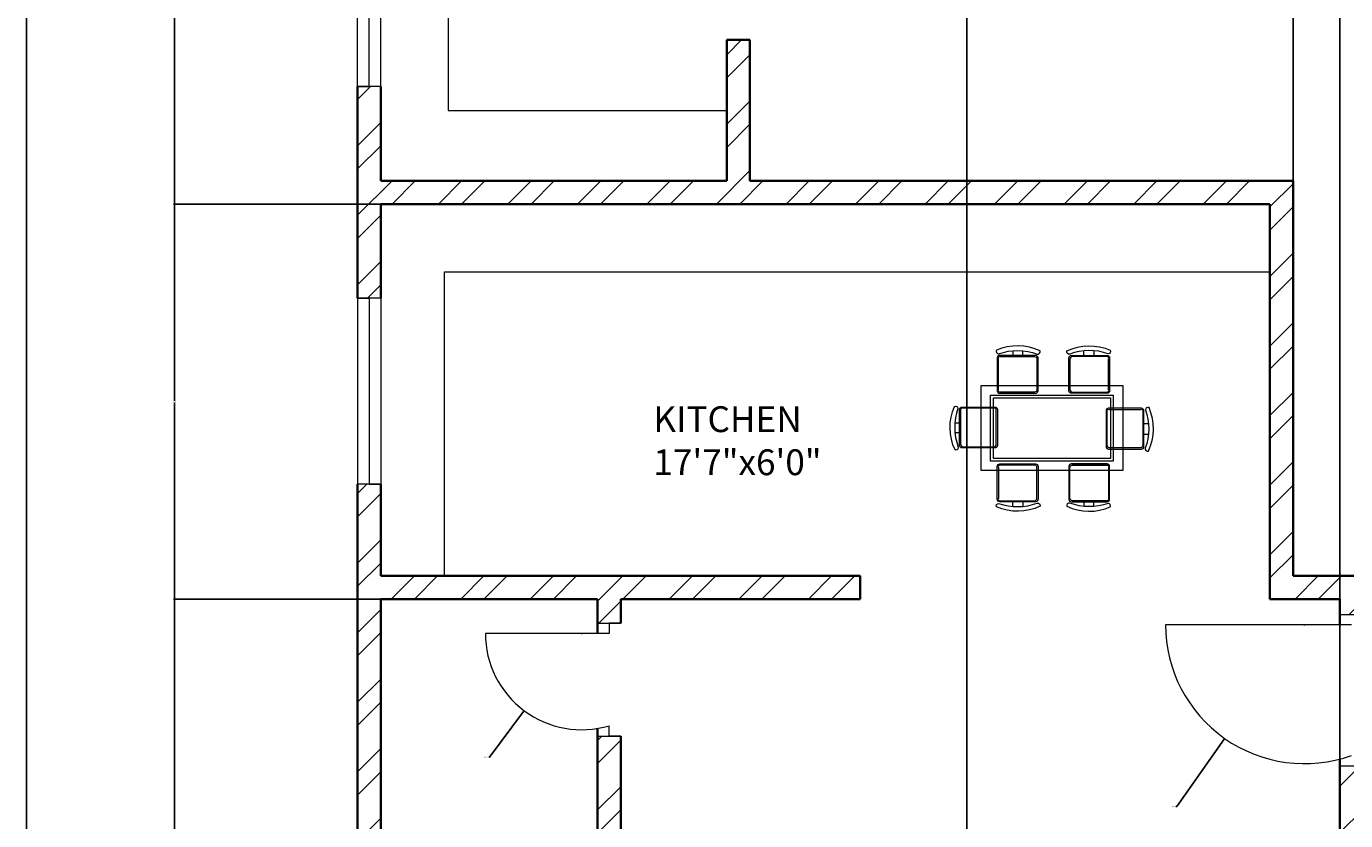
# Model space of a CAD drawing. Units: inches. Extents: x 2064 to 2782, y 1196 to 2299.
# Tile 3 of 11: x 2064 to 2320, y 1809 to 1963. Entities that reach past the tile are written whole.
import ezdxf

# ---------------------------------------------------------------- set-up
doc = ezdxf.new("R2010")
doc.units = ezdxf.units.IN
for name, color, linetype, lineweight in [('A-ANNO-DIMS', 2, 'Continuous', 18), ('A-ANNO-TTLB', 7, 'Continuous', 25), ('A-AREA-IDEN', 7, 'Continuous', 18), ('A-DOOR', 11, 'Continuous', 18), ('A-FLOR-CASE', 8, 'Continuous', 18), ('A-FURN', 8, 'Continuous', 13), ('A-GLAZ', 151, 'Continuous', 18), ('A-WALL', 7, 'Continuous', 35), ('A-WALL-PATT', 9, 'Continuous', 13)]:
    doc.layers.add(name, color=color, linetype=linetype, lineweight=lineweight)
doc.styles.get("Standard").update_dxf_attribs({"font": 'arial.ttf'})
doc.dimstyles.get("Standard").update_dxf_attribs({"dimtxt": 0.18, "dimasz": 0.18, "dimexe": 0.18, "dimexo": 0.0625, "dimgap": 0.09, "dimtad": 0, "dimtih": 1, "dimtoh": 1, "dimdec": 4, "dimzin": 0, "dimdsep": 46, "dimtxsty": 'Standard', "dimcen": 0.09, "dimadec": 0, "dimazin": 0, "dimtfac": 1, "dimtdec": 4, "dimtofl": 0, "dimtmove": 0, "dimatfit": 3, "dimfxl": 1, "dimtolj": 1, "dimtzin": 0, "dimarcsym": 0})

# ---------------------------------------------------------------- blocks, each defined once
blk = doc.blocks.new('WIN-36IN')
for p, q in [((0, 36), (4.5, 36)), ((0, 36), (0, 0)), ((4.5, 36), (2.25, 36)), ((2.25, 36), (2.25, 0)), ((4.5, 36), (4.5, 0)), ((2.25, 0), (0, 0)), ((0, 0), (4.5, 0))]:
    blk.add_line(p, q)
blk = doc.blocks.new('CHAIR-DINING')
for points in [[(7.35, 7.85, 0.414214), (6.87, 8.33), (0.49, 8.33, 0.414214), (0, 7.85), (0, 0.91, 0.414214), (0.49, 0.42), (6.87, 0.42, 0.414214), (7.35, 0.91), (7.35, 7.85)], [(7.35, 7.85, 0.414214), (6.87, 8.33), (0.49, 8.33, 0.414214), (0, 7.85), (0, 0.91, 0.414214), (0.49, 0.42), (6.87, 0.42, 0.414214), (7.35, 0.91), (7.35, 7.85)], [(7.65, 8.06, -0.175809), (7.6, 0.59, 0.578392), (8.22, 0.02, 0.214524), (8.33, 8.46, 0.552014), (7.65, 8.06, -0.065079)], [(7.65, 8.06, -0.175809), (7.6, 0.59, 0.578392), (8.22, 0.02, 0.214524), (8.33, 8.46, 0.552014), (7.65, 8.06, -0.065079)], [(7.35, 3.34), (8.23, 3.34, -0.064759)], [(7.35, 3.34), (8.23, 3.34, -0.064759)]]:
    blk.add_lwpolyline(points, format="xyb")
for points in [[(7.13, 7.84), (7.13, 1.13, -0.414214), (6.65, 0.64), (0.7, 0.64, -0.414214), (0.22, 1.13), (0.22, 7.84, -0.512069), (0.7, 8.11), (6.65, 8.11, -0.512069)], [(7.13, 7.84), (7.13, 1.12, -0.414214), (6.65, 0.64), (0.7, 0.64, -0.414214), (0.22, 1.12), (0.22, 7.84, -0.512069), (0.7, 8.11), (6.65, 8.11, -0.512069)]]:
    blk.add_lwpolyline(points, format="xyb", close=True)
blk.add_lwpolyline([(8.25, 5.29), (7.35, 5.29)])
blk.add_lwpolyline([(8.25, 5.29), (7.35, 5.29)])
blk = doc.blocks.new('TABLE-DINING')
for points in [[(0, 16.47), (27.45, 16.47), (27.45, 0), (0, 0)], [(0, 16.47), (27.45, 16.47), (27.45, 0), (0, 0)], [(1.83, 14.64), (25.62, 14.64), (25.62, 1.83), (1.83, 1.83)], [(1.83, 14.64), (25.62, 14.64), (25.62, 1.83), (1.83, 1.83)], [(2.38, 14.09), (25.07, 14.09), (25.07, 2.38), (2.38, 2.38)], [(2.38, 14.09), (25.07, 14.09), (25.07, 2.38), (2.38, 2.38)]]:
    blk.add_lwpolyline(points, close=True)
blk = doc.blocks.new('*D26')
at = {"layer": 'A-ANNO-DIMS', "color": 0, "lineweight": -2, "transparency": 16777216}
for p, q in [((2246.18, 1643.35), (2246.18, 2269.97)), ((2246.36, 2269.79), (2281.92, 2269.79)), ((2318.27, 2269.79), (2282.71, 2269.79)), ((2318.45, 1640.85), (2318.45, 2269.97))]:
    blk.add_line(p, q, dxfattribs=at)
at = {"layer": 'A-ANNO-DIMS', "color": 0, "transparency": 16777216}
for points in [[(2246.36, 2269.82), (2246.36, 2269.76), (2246.18, 2269.79)], [(2318.27, 2269.82), (2318.27, 2269.76), (2318.45, 2269.79)]]:
    blk.add_solid(points, dxfattribs=at)
at = {"layer": 'Defpoints', "color": 0, "transparency": 16777216}
for p in [(2318.45, 2269.79), (2246.18, 1643.29), (2318.45, 1640.79)]:
    blk.add_point(p, dxfattribs=at)
at = {"layer": 'A-ANNO-DIMS', "color": 0, "transparency": 16777216, "insert": (2282.32, 2269.79), "char_height": 0.18, "attachment_point": 5}
blk.add_mtext('\\A1;72.27', dxfattribs=at)
blk = doc.blocks.new('*D29')
at = {"layer": 'A-ANNO-DIMS', "color": 0, "lineweight": -2, "transparency": 16777216}
for p, q in [((2132.61, 1851.79), (2092.49, 1851.79)), ((2092.67, 1851.61), (2092.67, 1771.72)), ((2092.67, 1691.47), (2092.67, 1771.36)), ((2128.11, 1691.29), (2092.49, 1691.29))]:
    blk.add_line(p, q, dxfattribs=at)
at = {"layer": 'A-ANNO-DIMS', "color": 0, "transparency": 16777216}
for points in [[(2092.64, 1851.61), (2092.7, 1851.61), (2092.67, 1851.79)], [(2092.64, 1691.47), (2092.7, 1691.47), (2092.67, 1691.29)]]:
    blk.add_solid(points, dxfattribs=at)
at = {"layer": 'Defpoints', "color": 0, "transparency": 16777216}
for p in [(2092.67, 1851.79), (2132.67, 1851.79), (2128.17, 1691.29)]:
    blk.add_point(p, dxfattribs=at)
at = {"layer": 'A-ANNO-DIMS', "color": 0, "transparency": 16777216, "insert": (2092.67, 1771.54), "char_height": 0.18, "attachment_point": 5}
blk.add_mtext('\\A1;160.5', dxfattribs=at)
blk = doc.blocks.new('*D30')
at = {"layer": 'A-ANNO-DIMS', "color": 0, "lineweight": -2, "transparency": 16777216}
for p, q in [((2132.61, 1928.29), (2092.49, 1928.29)), ((2092.67, 1928.11), (2092.67, 1890.22)), ((2092.67, 1851.97), (2092.67, 1889.86)), ((2132.61, 1851.79), (2092.49, 1851.79))]:
    blk.add_line(p, q, dxfattribs=at)
at = {"layer": 'A-ANNO-DIMS', "color": 0, "transparency": 16777216}
for points in [[(2092.64, 1928.11), (2092.7, 1928.11), (2092.67, 1928.29)], [(2092.64, 1851.97), (2092.7, 1851.97), (2092.67, 1851.79)]]:
    blk.add_solid(points, dxfattribs=at)
at = {"layer": 'Defpoints', "color": 0, "transparency": 16777216}
for p in [(2092.67, 1928.29), (2132.67, 1928.29), (2132.67, 1851.79)]:
    blk.add_point(p, dxfattribs=at)
at = {"layer": 'A-ANNO-DIMS', "color": 0, "transparency": 16777216, "insert": (2092.67, 1890.04), "char_height": 0.18, "attachment_point": 5}
blk.add_mtext('\\A1;76.5', dxfattribs=at)
blk = doc.blocks.new('*D31')
at = {"layer": 'A-ANNO-DIMS', "color": 0, "lineweight": -2, "transparency": 16777216}
for p, q in [((2132.61, 2004.79), (2092.49, 2004.79)), ((2092.67, 2004.61), (2092.67, 1966.72)), ((2092.67, 1928.47), (2092.67, 1966.36)), ((2132.61, 1928.29), (2092.49, 1928.29))]:
    blk.add_line(p, q, dxfattribs=at)
at = {"layer": 'A-ANNO-DIMS', "color": 0, "transparency": 16777216}
for points in [[(2092.64, 2004.61), (2092.7, 2004.61), (2092.67, 2004.79)], [(2092.64, 1928.47), (2092.7, 1928.47), (2092.67, 1928.29)]]:
    blk.add_solid(points, dxfattribs=at)
at = {"layer": 'Defpoints', "color": 0, "transparency": 16777216}
for p in [(2092.67, 2004.79), (2132.67, 2004.79), (2132.67, 1928.29)]:
    blk.add_point(p, dxfattribs=at)
at = {"layer": 'A-ANNO-DIMS', "color": 0, "transparency": 16777216, "insert": (2092.67, 1966.54), "char_height": 0.18, "attachment_point": 5}
blk.add_mtext('\\A1;76.5', dxfattribs=at)
blk = doc.blocks.new('*D35')
at = {"layer": 'A-ANNO-DIMS', "color": 0, "lineweight": -2, "transparency": 16777216}
for p, q in [((2309.4, 1932.85), (2309.4, 2269.97)), ((2309.58, 2269.79), (2347.37, 2269.79)), ((2385.94, 2269.79), (2348.16, 2269.79)), ((2386.12, 1856.35), (2386.12, 2269.97))]:
    blk.add_line(p, q, dxfattribs=at)
at = {"layer": 'A-ANNO-DIMS', "color": 0, "transparency": 16777216}
for points in [[(2309.58, 2269.82), (2309.58, 2269.76), (2309.4, 2269.79)], [(2385.94, 2269.82), (2385.94, 2269.76), (2386.12, 2269.79)]]:
    blk.add_solid(points, dxfattribs=at)
at = {"layer": 'Defpoints', "color": 0, "transparency": 16777216}
for p in [(2386.12, 2269.79), (2309.4, 1932.79), (2386.12, 1856.29)]:
    blk.add_point(p, dxfattribs=at)
at = {"layer": 'A-ANNO-DIMS', "color": 0, "transparency": 16777216, "insert": (2347.76, 2269.79), "char_height": 0.18, "attachment_point": 5}
blk.add_mtext('\\A1;76.72', dxfattribs=at)
blk = doc.blocks.new('*D47')
at = {"layer": 'A-ANNO-DIMS', "color": 0, "lineweight": -2, "transparency": 16777216}
for p, q in [((2311.51, 1846.83), (2311.69, 1846.83)), ((2311.6, 1846.74), (2311.6, 1846.92)), ((2286.85, 1811.62), (2296.03, 1824.68)), ((2286.67, 1811.62), (2286.85, 1811.62))]:
    blk.add_line(p, q, dxfattribs=at)
at = {"layer": 'A-ANNO-DIMS', "color": 0, "transparency": 16777216}
blk.add_solid([(2296, 1824.7), (2296.05, 1824.66), (2296.13, 1824.83)], dxfattribs=at)
at = {"layer": 'Defpoints', "color": 0, "transparency": 16777216}
for p in [(2311.6, 1846.83), (2296.13, 1824.83)]:
    blk.add_point(p, dxfattribs=at)
at = {"layer": 'A-ANNO-DIMS', "color": 0, "transparency": 16777216, "insert": (2286.26, 1811.62), "char_height": 0.18, "attachment_point": 5}
blk.add_mtext('\\A1;R26.9', dxfattribs=at)
blk = doc.blocks.new('*D49')
at = {"layer": 'A-ANNO-DIMS', "color": 0, "lineweight": -2, "transparency": 16777216}
for p, q in [((2171.48, 1845.15), (2171.66, 1845.15)), ((2171.57, 1845.06), (2171.57, 1845.24)), ((2153.75, 1821.21), (2160.33, 1830.04)), ((2153.57, 1821.21), (2153.75, 1821.21))]:
    blk.add_line(p, q, dxfattribs=at)
at = {"layer": 'A-ANNO-DIMS', "color": 0, "transparency": 16777216}
blk.add_solid([(2160.3, 1830.06), (2160.35, 1830.02), (2160.43, 1830.19)], dxfattribs=at)
at = {"layer": 'Defpoints', "color": 0, "transparency": 16777216}
for p in [(2171.57, 1845.15), (2160.43, 1830.19)]:
    blk.add_point(p, dxfattribs=at)
at = {"layer": 'A-ANNO-DIMS', "color": 0, "transparency": 16777216, "insert": (2153.02, 1821.21), "char_height": 0.18, "attachment_point": 5}
blk.add_mtext('\\A1;R18.648', dxfattribs=at)

msp = doc.modelspace()

# ---------------------------------------------------------------- hatches: boundary and pattern name
at = {"layer": 'A-WALL-PATT'}
h = msp.add_hatch(dxfattribs=at)
h.set_pattern_fill('ANSI32', color=256)
h.paths.add_polyline_path([(2489.7688, 2189.2917), (2574.5454, 2189.2917), (2574.5454, 2191.5417), (2574.5454, 2193.7917), (2570.6691, 2193.7917), (2570.6691, 2197.3052), (2568.4191, 2197.3052), (2566.1691, 2197.3052), (2566.1691, 2193.7917), (2494.1691, 2193.7917), (2494.1691, 2229.7917), (2523.2441, 2229.7917), (2523.2441, 2234.2917), (2471.2886, 2234.2917), (2471.2886, 2229.7917), (2489.6691, 2229.7917), (2489.6691, 2193.7917), (2417.6691, 2193.7917), (2417.6691, 2197.0632), (2415.4191, 2197.0632), (2413.1691, 2197.0632), (2413.1691, 2193.7917), (2406.8865, 2193.7917), (2406.8865, 2189.2917), (2485.2688, 2189.2917), (2485.2688, 2063.2917), (2369.1629, 2063.2917), (2369.1629, 2058.7917), (2386.1222, 2058.7917), (2386.1222, 1856.2917), (2382.1576, 1856.2917), (2382.1576, 1851.7917), (2394.9764, 1851.7917), (2394.9764, 1854.0417), (2394.9764, 1856.2917), (2390.6222, 1856.2917), (2390.6222, 2058.7917), (2485.2688, 2058.7917), (2493.762, 2058.7917), (2493.762, 2061.0417), (2493.762, 2063.2917), (2489.7688, 2063.2917)])
h.paths.add_polyline_path([(2447.2886, 2234.2917), (2413.1691, 2234.2917), (2413.1691, 2217.3799), (2417.6691, 2217.3799), (2417.6691, 2229.7917), (2447.2886, 2229.7917)], flags=17)
h.paths.add_polyline_path([(2570.6691, 2234.2917), (2547.2441, 2234.2917), (2547.2441, 2229.7917), (2566.1691, 2229.7917), (2566.1691, 2216.5615), (2570.6691, 2216.5615)], flags=17)
h.paths.add_polyline_path([(2653.1691, 2189.2917), (2653.1691, 2193.7917), (2640.8843, 2193.7917), (2640.8843, 2189.2917), (2648.6691, 2189.2917), (2648.6691, 2162.7138), (2653.1691, 2162.7138)])
h.paths.add_polyline_path([(2653.1691, 2102.7138), (2648.6691, 2102.7138), (2648.6691, 2063.2917), (2526.7281, 2063.2917), (2526.7281, 2058.7917), (2541.1691, 2058.7917), (2541.1691, 1993.2917), (2545.6691, 1993.2917), (2545.6691, 1997.7917), (2545.6691, 2058.7917), (2648.6691, 2058.7917), (2648.6691, 2050.1099), (2653.1691, 2050.1099)])
h.paths.add_polyline_path([(2600.6691, 1856.2917), (2493.4607, 1856.2917), (2493.4607, 1851.7917), (2596.1691, 1851.7917), (2596.1691, 1695.7917), (2594.0816, 1695.7917), (2594.0816, 1691.2917), (2614.7905, 1691.2917), (2614.7905, 1645.2917), (2536.7905, 1645.2917), (2536.7905, 1691.2917), (2539.332, 1691.2917), (2539.332, 1693.5417), (2539.332, 1695.7917), (2452.1691, 1695.7917), (2452.1691, 1851.7917), (2456.0775, 1851.7917), (2456.0775, 1856.2917), (2427.1536, 1856.2917), (2427.1536, 1851.7917), (2447.6691, 1851.7917), (2447.6691, 1695.7917), (2447.6691, 1645.2917), (2405.1469, 1645.2917), (2405.1469, 1640.7917), (2452.1691, 1640.7917), (2452.1691, 1645.2917), (2452.1691, 1691.2917), (2534.7905, 1691.2917), (2534.7905, 1645.2917), (2534.7905, 1643.2917), (2614.7905, 1643.2917), (2616.7905, 1643.2917), (2616.7905, 1691.2917), (2622.4029, 1691.2917), (2622.4029, 1693.7143), (2622.4029, 1695.7917), (2600.6691, 1695.7917), (2600.6691, 1779.7917), (2648.6691, 1779.7917), (2648.6691, 1695.7917), (2646.4029, 1695.7917), (2646.4029, 1691.2917), (2653.1691, 1691.2917), (2653.1691, 1906.3508), (2648.6691, 1906.3508), (2648.6691, 1856.2917), (2648.6691, 1784.2917), (2600.6691, 1784.2917)])
h.paths.add_polyline_path([(2322.9532, 1819.5181), (2320.7032, 1819.5181), (2318.4532, 1819.5181), (2318.4532, 1695.7917), (2242.7664, 1695.7917), (2242.7664, 1691.2917), (2318.4532, 1691.2917), (2318.4532, 1640.7917), (2322.9532, 1640.7917), (2345.1469, 1640.7917), (2345.1469, 1643.0417), (2345.1469, 1645.2917), (2322.9532, 1645.2917), (2322.9532, 1691.2917), (2322.9532, 1695.7917)])
h.paths.add_polyline_path([(2166.1825, 1691.2917), (2164.1825, 1691.2917), (2164.1825, 1643.2917), (2166.1825, 1643.2917), (2246.1825, 1643.2917), (2246.1825, 1645.2917), (2246.1825, 1691.2917), (2244.1825, 1691.2917), (2244.1825, 1645.2917), (2166.1825, 1645.2917)])
h.paths.add_polyline_path([(2309.404, 1932.7917), (2204.1691, 1932.7917), (2204.1691, 1960.0962), (2199.6691, 1960.0962), (2199.6691, 1932.7917), (2132.6691, 1932.7917), (2132.6691, 1951.0737), (2128.1691, 1951.0737), (2128.1691, 1910.0412), (2132.6691, 1910.0412), (2132.6691, 1928.2917), (2304.904, 1928.2917), (2304.904, 1856.2917), (2304.904, 1851.7917), (2318.4532, 1851.7917), (2318.4532, 1848.8308), (2322.9532, 1848.8308), (2322.9532, 1851.7917), (2347.7631, 1851.7917), (2347.7631, 1856.2917), (2309.404, 1856.2917)])
h.paths.add_polyline_path([(2132.6691, 2044.9092), (2130.4191, 2044.9092), (2128.1691, 2044.9092), (2128.1691, 1987.0737), (2132.6691, 1987.0737), (2132.6691, 2004.7917), (2199.6691, 2004.7917), (2204.1691, 2004.7917), (2204.1691, 2009.2917), (2132.6691, 2009.2917)])
h.paths.add_polyline_path([(2186.6691, 2195.9329), (2184.4191, 2195.9329), (2184.4191, 2195.8929), (2182.1691, 2195.9329), (2182.1691, 2193.7917), (2128.1691, 2193.7917), (2128.1691, 2181.4967), (2132.6691, 2181.4967), (2132.6691, 2182.7769), (2132.6691, 2189.2917), (2182.1691, 2189.2917), (2182.1691, 2135.2917), (2179.804, 2135.2917), (2179.804, 2130.7917), (2190.215, 2130.7917), (2190.215, 2133.0417), (2190.215, 2135.2917), (2186.6691, 2135.2917)])
h.paths.add_polyline_path([(2340.0628, 2189.2917), (2340.0628, 2191.5417), (2340.0628, 2193.7917), (2335.1691, 2193.7917), (2335.1691, 2234.2917), (2280.6746, 2234.2917), (2280.6746, 2229.7917), (2330.6691, 2229.7917), (2330.6691, 2193.7917), (2330.6691, 2135.2917), (2218.6309, 2135.2917), (2218.6309, 2130.7917), (2330.7688, 2130.7917), (2330.7688, 2008.4023), (2335.2688, 2008.4023), (2335.2688, 2058.7917), (2338.9208, 2058.7917), (2338.9208, 2061.0417), (2338.9208, 2063.2917), (2335.2688, 2063.2917), (2335.2688, 2189.2917)])
h.paths.add_polyline_path([(2220.6746, 2234.2917), (2182.1691, 2234.2917), (2182.1691, 2227.4187), (2186.6691, 2227.4187), (2186.6691, 2229.7917), (2220.6746, 2229.7917), (2220.6746, 2232.0417)])
h.paths.add_polyline_path([(2158.8146, 2135.2917), (2132.6691, 2135.2917), (2132.6691, 2157.4967), (2128.1691, 2157.4967), (2128.1691, 2104.9092), (2132.6691, 2104.9092), (2132.6691, 2130.7917), (2158.8146, 2130.7917), (2158.8146, 2133.0417)])
h.paths.add_polyline_path([(2396.0464, 2062.2045), (2434.8868, 2062.2045), (2434.8868, 2080.8619), (2396.0464, 2080.8619)], flags=24)
h.paths.add_polyline_path([(2196.1396, 1653.3449), (2232.023, 1653.3449), (2232.023, 1672.0022), (2196.1396, 1672.0022)], flags=25)
h = msp.add_hatch(dxfattribs=at)
h.set_pattern_fill('ANSI32', color=256)
h.paths.add_polyline_path([(2225.5529, 1856.2917), (2132.6691, 1856.2917), (2132.6691, 1874.0412), (2130.4191, 1874.0412), (2128.1691, 1874.0412), (2128.1691, 1691.2917), (2136.6659, 1691.2917), (2136.6659, 1693.5417), (2136.6659, 1695.7917), (2132.6691, 1695.7917), (2132.6691, 1851.7917), (2174.6691, 1851.7917), (2174.6691, 1847.1454), (2179.1691, 1847.1454), (2179.1691, 1851.7917), (2225.5529, 1851.7917)])
h.paths.add_polyline_path([(2179.1691, 1825.2823), (2176.9191, 1825.2823), (2174.6691, 1825.2823), (2174.6691, 1695.7917), (2160.6659, 1695.7917), (2160.6659, 1691.2917), (2182.0177, 1691.2917), (2182.0177, 1693.5417), (2182.0177, 1695.7917), (2179.1691, 1695.7917)], flags=17)

# ---------------------------------------------------------------- linework, layer by layer
at = {"layer": 'A-ANNO-TTLB'}
msp.add_lwpolyline([(2063.9994, 2298.574), (2782.0941, 2298.574), (2782.0941, 1490.6238), (2063.9994, 1490.6238)], close=True, dxfattribs=at)
at = {"layer": 'A-DOOR'}
for p, q in [((2318.4532, 1848.8308), (2322.9532, 1848.8308)), ((2174.6691, 1847.1454), (2179.1691, 1847.1454)), ((2179.1691, 1847.1454), (2176.9191, 1847.1454)), ((2176.9191, 1847.1454), (2176.9191, 1845.1454)), ((2320.7032, 1846.8308), (2284.7032, 1846.8308)), ((2176.9191, 1845.1454), (2152.9191, 1845.1454)), ((2174.6691, 1825.2823), (2179.1691, 1825.2823)), ((2176.9191, 1825.2823), (2176.9191, 1827.2823)), ((2179.1691, 1825.2823), (2176.9191, 1825.2823)), ((2318.4532, 1819.5181), (2322.9532, 1819.5181))]:
    msp.add_line(p, q, dxfattribs=at)
for centre, radius, end in [((2311.6023, 1846.8308), 26.8991, 289.775476), ((2171.5668, 1845.1454), 18.6477, 286.679623)]:
    msp.add_arc(centre, radius, 180, end, dxfattribs=at)
at = {"layer": 'A-FLOR-CASE'}
for p, q in [((2145.6809, 2004.7917), (2145.6809, 1946.3811)), ((2145.6809, 1946.3811), (2199.6691, 1946.3811)), ((2145.0217, 1856.2917), (2145.0217, 1915.1527)), ((2145.0217, 1915.1527), (2304.904, 1915.1527))]:
    msp.add_line(p, q, dxfattribs=at)
at = {"layer": 'A-FURN'}
for points in [[(2252.3508, 1899.2968, -0.17580919), (2259.8263, 1899.2402, 0.57839206), (2260.3926, 1899.8629, 0.21452438), (2251.9544, 1899.9761, 0.55201397), (2252.3508, 1899.2968, -0.06507904)], [(2252.3508, 1899.2965, -0.17580919), (2259.8263, 1899.2399, 0.57839206), (2260.3926, 1899.8626, 0.21452438), (2251.9544, 1899.9758, 0.55201397), (2252.3508, 1899.2965, -0.06507904)], [(2259.5091, 1898.9968), (2252.5692, 1898.9968, 0.41421356), (2252.0836, 1898.5113), (2252.0836, 1892.1301, 0.41421356), (2252.5692, 1891.6446), (2259.5091, 1891.6446, 0.41421356), (2259.9946, 1892.1301), (2259.9946, 1898.5113, 0.41421356), (2259.5091, 1898.9968)], [(2259.5091, 1898.9965), (2252.5692, 1898.9965, 0.41421356), (2252.0837, 1898.511), (2252.0837, 1892.1298, 0.41421356), (2252.5692, 1891.6443), (2259.5091, 1891.6443, 0.41421356), (2259.9947, 1892.1298), (2259.9947, 1898.511, 0.41421356), (2259.5091, 1898.9965)], [(2257.0715, 1898.9968), (2257.0715, 1899.8745, -0.06475861)], [(2257.0715, 1898.9965), (2257.0715, 1899.8742, -0.06475861)], [(2266.1196, 1899.2402, -0.57839206), (2265.5533, 1899.8629, -0.21452438), (2273.9915, 1899.9761, -0.55201397), (2273.5951, 1899.2968, 0.1758092), (2266.1196, 1899.2402)], [(2266.1196, 1899.2399, -0.57839206), (2265.5533, 1899.8626, -0.21452438), (2273.9915, 1899.9758, -0.55201397), (2273.5951, 1899.2965, 0.1758092), (2266.1196, 1899.2399)], [(2273.3767, 1898.9968, -0.41421356), (2273.8622, 1898.5113), (2273.8622, 1892.1301, -0.41421356), (2273.3767, 1891.6446), (2266.4368, 1891.6446, -0.41421356), (2265.9512, 1892.1301), (2265.9512, 1898.5113, -0.41421356), (2266.4368, 1898.9968), (2273.3767, 1898.9968)], [(2273.3767, 1898.9965, -0.41421356), (2273.8623, 1898.511), (2273.8623, 1892.1298, -0.41421356), (2273.3767, 1891.6443), (2266.4368, 1891.6443, -0.41421356), (2265.9513, 1892.1298), (2265.9513, 1898.511, -0.41421356), (2266.4368, 1898.9965), (2273.3767, 1898.9965)], [(2268.8744, 1898.9968), (2268.8744, 1899.8745, 0.06475861)], [(2268.8744, 1898.9965), (2268.8744, 1899.8742, 0.06475861)], [(2244.5301, 1881.2448, -0.57839206), (2243.9074, 1880.6784, -0.21452438), (2243.7942, 1889.1166, -0.55201397), (2244.4735, 1888.7202, 0.17580937), (2244.5301, 1881.2448)], [(2244.5301, 1881.2445, -0.57839206), (2243.9074, 1880.6782, -0.21452438), (2243.7942, 1889.1163, -0.55201397), (2244.4735, 1888.7199, 0.17580937), (2244.5301, 1881.2445)], [(2244.7735, 1888.5019, -0.41421356), (2245.259, 1888.9874), (2251.6402, 1888.9874, -0.41421356), (2252.1257, 1888.5019), (2252.1257, 1881.5619, -0.41421356), (2251.6402, 1881.0764), (2245.259, 1881.0764, -0.41421356), (2244.7735, 1881.5619), (2244.7735, 1888.5019)], [(2244.7735, 1888.5016, -0.41421356), (2245.259, 1888.9871), (2251.6402, 1888.9871, -0.41421356), (2252.1257, 1888.5016), (2252.1257, 1881.5616, -0.41421356), (2251.6402, 1881.0761), (2245.259, 1881.0761, -0.41421356), (2244.7735, 1881.5616), (2244.7735, 1888.5016)], [(2244.7735, 1883.9996), (2243.8958, 1883.9996, 0.06475861)], [(2244.7735, 1883.9993), (2243.8958, 1883.9993, 0.06475861)], [(2259.5091, 1870.631), (2252.5692, 1870.631, -0.41421356), (2252.0836, 1871.1166), (2252.0836, 1877.4977, -0.41421356), (2252.5692, 1877.9832), (2259.5091, 1877.9832, -0.41421356), (2259.9946, 1877.4977), (2259.9946, 1871.1166, -0.41421356), (2259.5091, 1870.631)], [(2259.5091, 1870.6307), (2252.5692, 1870.6307, -0.41421356), (2252.0837, 1871.1163), (2252.0837, 1877.4974, -0.41421356), (2252.5692, 1877.9829), (2259.5091, 1877.9829, -0.41421356), (2259.9947, 1877.4974), (2259.9947, 1871.1163, -0.41421356), (2259.5091, 1870.6307)], [(2273.3767, 1870.631, 0.41421356), (2273.8622, 1871.1166), (2273.8622, 1877.4977, 0.41421356), (2273.3767, 1877.9832), (2266.4368, 1877.9832, 0.41421356), (2265.9512, 1877.4977), (2265.9512, 1871.1166, 0.41421356), (2266.4368, 1870.631), (2273.3767, 1870.631)], [(2273.3767, 1870.6307, 0.41421356), (2273.8623, 1871.1163), (2273.8623, 1877.4974, 0.41421356), (2273.3767, 1877.9829), (2266.4368, 1877.9829, 0.41421356), (2265.9513, 1877.4974), (2265.9513, 1871.1163, 0.41421356), (2266.4368, 1870.6307), (2273.3767, 1870.6307)], [(2259.8263, 1870.3876, -0.57839206), (2260.3926, 1869.7649, -0.21452438), (2251.9544, 1869.6517, -0.55201397), (2252.3508, 1870.331, 0.17580929), (2259.8263, 1870.3876)], [(2259.8263, 1870.3873, -0.57839206), (2260.3926, 1869.7646, -0.21452438), (2251.9544, 1869.6514, -0.55201397), (2252.3508, 1870.3307, 0.17580929), (2259.8263, 1870.3873)], [(2257.0715, 1870.631), (2257.0715, 1869.7533, 0.06475861)], [(2257.0715, 1870.6307), (2257.0715, 1869.7531, 0.06475861)], [(2273.5951, 1870.331, -0.17580928), (2266.1196, 1870.3876, 0.57839206), (2265.5533, 1869.7649, 0.21452438), (2273.9915, 1869.6517, 0.55201397), (2273.5951, 1870.331, -0.06507904)], [(2273.5951, 1870.3307, -0.17580928), (2266.1196, 1870.3873, 0.57839206), (2265.5533, 1869.7646, 0.21452438), (2273.9915, 1869.6514, 0.55201397), (2273.5951, 1870.3307, -0.06507904)], [(2268.8744, 1870.631), (2268.8744, 1869.7533, -0.06475861)], [(2268.8744, 1870.6307), (2268.8744, 1869.7531, -0.06475861)]]:
    msp.add_lwpolyline(points, format="xyb", dxfattribs=at)
for points in [[(2255.1289, 1899.8904), (2255.1289, 1898.9968)], [(2255.1289, 1899.8901), (2255.1289, 1898.9965)], [(2270.817, 1899.8904), (2270.817, 1898.9968)], [(2270.817, 1899.8901), (2270.817, 1898.9965)], [(2243.8799, 1885.9422), (2244.7735, 1885.9422)], [(2243.8799, 1885.9419), (2244.7735, 1885.9419)], [(2255.1289, 1869.7374), (2255.1289, 1870.631)], [(2255.1289, 1869.7371), (2255.1289, 1870.6307)], [(2270.817, 1869.7374), (2270.817, 1870.631)], [(2270.817, 1869.7371), (2270.817, 1870.6307)]]:
    msp.add_lwpolyline(points, dxfattribs=at)
for points in [[(2252.5721, 1898.778), (2259.2904, 1898.778, -0.41421356), (2259.7759, 1898.2925), (2259.7759, 1892.3488, -0.41421356), (2259.2904, 1891.8633), (2252.5721, 1891.8633, -0.51206948), (2252.3024, 1892.3488), (2252.3024, 1898.2925, -0.51206948)], [(2252.5721, 1898.7778), (2259.2904, 1898.7778, -0.41421356), (2259.7759, 1898.2922), (2259.7759, 1892.3486, -0.41421356), (2259.2904, 1891.863), (2252.5721, 1891.863, -0.51206948), (2252.3024, 1892.3486), (2252.3024, 1898.2922, -0.51206948)], [(2273.3738, 1898.778), (2266.6555, 1898.778, 0.41421356), (2266.17, 1898.2925), (2266.17, 1892.3488, 0.41421356), (2266.6555, 1891.8633), (2273.3738, 1891.8633, 0.51206948), (2273.6435, 1892.3488), (2273.6435, 1898.2925, 0.51206948)], [(2273.3738, 1898.7778), (2266.6555, 1898.7778, 0.41421356), (2266.17, 1898.2922), (2266.17, 1892.3486, 0.41421356), (2266.6555, 1891.863), (2273.3738, 1891.863, 0.51206948), (2273.6435, 1892.3486), (2273.6435, 1898.2922, 0.51206948)], [(2244.9922, 1888.4989), (2244.9922, 1881.7806, 0.41421356), (2245.4778, 1881.2951), (2251.4214, 1881.2951, 0.41421356), (2251.907, 1881.7806), (2251.907, 1888.4989, 0.51206948), (2251.4214, 1888.7686), (2245.4778, 1888.7686, 0.51206948)], [(2244.9923, 1888.4986), (2244.9923, 1881.7804, 0.41421356), (2245.4778, 1881.2948), (2251.4215, 1881.2948, 0.41421356), (2251.907, 1881.7804), (2251.907, 1888.4986, 0.51206948), (2251.4215, 1888.7684), (2245.4778, 1888.7684, 0.51206948)], [(2252.5721, 1870.8498), (2259.2904, 1870.8498, 0.41421356), (2259.7759, 1871.3353), (2259.7759, 1877.279, 0.41421356), (2259.2904, 1877.7645), (2252.5721, 1877.7645, 0.51206948), (2252.3024, 1877.279), (2252.3024, 1871.3353, 0.51206948)], [(2252.5721, 1870.8495), (2259.2904, 1870.8495, 0.41421356), (2259.7759, 1871.335), (2259.7759, 1877.2787, 0.41421356), (2259.2904, 1877.7642), (2252.5721, 1877.7642, 0.51206948), (2252.3024, 1877.2787), (2252.3024, 1871.335, 0.51206948)], [(2273.3738, 1870.8498), (2266.6555, 1870.8498, -0.41421356), (2266.17, 1871.3353), (2266.17, 1877.279, -0.41421356), (2266.6555, 1877.7645), (2273.3738, 1877.7645, -0.51206948), (2273.6435, 1877.279), (2273.6435, 1871.3353, -0.51206948)], [(2273.3738, 1870.8495), (2266.6555, 1870.8495, -0.41421356), (2266.17, 1871.335), (2266.17, 1877.2787, -0.41421356), (2266.6555, 1877.7642), (2273.3738, 1877.7642, -0.51206948), (2273.6435, 1877.2787), (2273.6435, 1871.335, -0.51206948)]]:
    msp.add_lwpolyline(points, format="xyb", close=True, dxfattribs=at)
at = {"layer": 'A-WALL'}
for p, q in [((2199.6691, 1960.0962), (2199.6691, 1932.7917)), ((2199.6691, 1960.0962), (2204.1691, 1960.0962)), ((2204.1691, 1960.0962), (2204.1691, 1932.7917)), ((2128.1691, 1951.0737), (2128.1691, 1910.0412)), ((2132.6691, 1951.0737), (2132.6691, 1932.7917)), ((2132.6691, 1932.7917), (2199.6691, 1932.7917)), ((2204.1691, 1932.7917), (2309.404, 1932.7917)), ((2309.404, 1856.2917), (2309.404, 1932.7917)), ((2132.6691, 1928.2917), (2304.904, 1928.2917)), ((2132.6691, 1928.2917), (2132.6691, 1910.0412)), ((2304.904, 1928.2917), (2304.904, 1856.2917)), ((2304.904, 1928.2917), (2304.904, 1856.2917)), ((2128.1691, 1874.0412), (2128.1691, 1691.2917)), ((2132.6691, 1874.0412), (2132.6691, 1856.2917)), ((2225.5529, 1856.2917), (2132.6691, 1856.2917)), ((2225.5529, 1856.2917), (2225.5529, 1851.7917)), ((2304.904, 1856.2917), (2304.904, 1851.7917)), ((2349.4652, 1856.2917), (2309.404, 1856.2917)), ((2132.6691, 1851.7917), (2174.6691, 1851.7917)), ((2132.6691, 1851.7917), (2132.6691, 1695.7917)), ((2174.6691, 1851.7917), (2174.6691, 1845.1454)), ((2179.1691, 1851.7917), (2179.1691, 1847.1454)), ((2179.1691, 1851.7917), (2225.5529, 1851.7917)), ((2304.904, 1851.7917), (2318.4532, 1851.7917)), ((2318.4532, 1846.8308), (2318.4532, 1851.7917)), ((2174.6691, 1826.7576), (2174.6691, 1695.7917)), ((2179.1691, 1825.2823), (2179.1691, 1695.7917)), ((2318.4532, 1695.7917), (2318.4532, 1820.8188))]:
    msp.add_line(p, q, dxfattribs=at)

# ---------------------------------------------------------------- block references
at = {"layer": 'A-FURN'}
for name, p in [('TABLE-DINING', (2248.9561, 1876.6681)), ('CHAIR-DINING', (2273.1588, 1880.4177))]:
    msp.add_blockref(name, p, dxfattribs=at)
at = {"layer": 'A-GLAZ', "rotation": 180}
msp.add_blockref('WIN-36IN', (2132.6691, 1987.0737), dxfattribs=at)
at = {"layer": 'A-GLAZ', "extrusion": (0, 0, -1), "zscale": -1}
msp.add_blockref('WIN-36IN', (-2132.6691, 1874.0412), dxfattribs=at)

# ---------------------------------------------------------------- texts
at = {"layer": 'A-AREA-IDEN', "insert": (2185.463, 1889.1359), "char_height": 5, "attachment_point": 1}
msp.add_mtext_dynamic_manual_height_columns('KITCHEN\\P17\'7"x6\'0"', width=276.208834, gutter_width=12.5, heights=[0], dxfattribs=at)

# ---------------------------------------------------------------- dimensions: what is measured, and where the dimension line sits
at = {"layer": 'A-ANNO-DIMS'}
for base, p1, p2, picture, middle in [((2318.4532, 2269.7917), (2246.1825, 1643.2917), (2318.4532, 1640.7917), '*D26', (2282.3178, 2269.7917)), ((2386.1222, 2269.7917), (2309.404, 1932.7917), (2386.1222, 1856.2917), '*D35', (2347.7631, 2269.7917))]:
    dim = msp.add_linear_dim(base=base, p1=p1, p2=p2, dimstyle='Standard', override={"dimdec": 2, "dimlfac": 1, "dimrnd": 0, "dimzin": 0, "dimdsep": 46, "dimlunit": 2}, dxfattribs=at)
    dim.commit()
    dim.dimension.update_dxf_attribs({"geometry": picture, "text_midpoint": middle})
for base, p1, p2, picture, middle in [((2092.6691, 2004.7917), (2132.6691, 1928.2917), (2132.6691, 2004.7917), '*D31', (2092.6691, 1966.5417)), ((2092.6691, 1928.2917), (2132.6691, 1851.7917), (2132.6691, 1928.2917), '*D30', (2092.6691, 1890.0417)), ((2092.6691, 1851.7917), (2128.1691, 1691.2917), (2132.6691, 1851.7917), '*D29', (2092.6691, 1771.5417))]:
    dim = msp.add_linear_dim(base=base, p1=p1, p2=p2, angle=90, dimstyle='Standard', override={"dimdec": 1, "dimlfac": 1, "dimrnd": 0, "dimzin": 0, "dimdsep": 46, "dimlunit": 2}, dxfattribs=at)
    dim.commit()
    dim.dimension.update_dxf_attribs({"geometry": picture, "text_midpoint": middle})
for center, mpoint, override, picture, middle in [((2311.6023, 1846.8308), (2296.13, 1824.827), {"dimdec": 1, "dimlfac": 1, "dimrnd": 0, "dimzin": 0, "dimdsep": 46, "dimlunit": 2}, '*D47', (2286.2565, 1811.6247)), ((2171.5668, 1845.1454), (2160.4331, 1830.1862), {"dimdec": 3, "dimlfac": 1, "dimrnd": 0, "dimzin": 0, "dimdsep": 46, "dimlunit": 2}, '*D49', (2153.023, 1821.2106))]:
    dim = msp.add_radius_dim(center=center, mpoint=mpoint, dimstyle='Standard', override=override, dxfattribs=at)
    dim.commit()
    dim.dimension.update_dxf_attribs({"geometry": picture, "text_midpoint": middle, "dimtype": 164})

doc.saveas('drawing.dxf')
